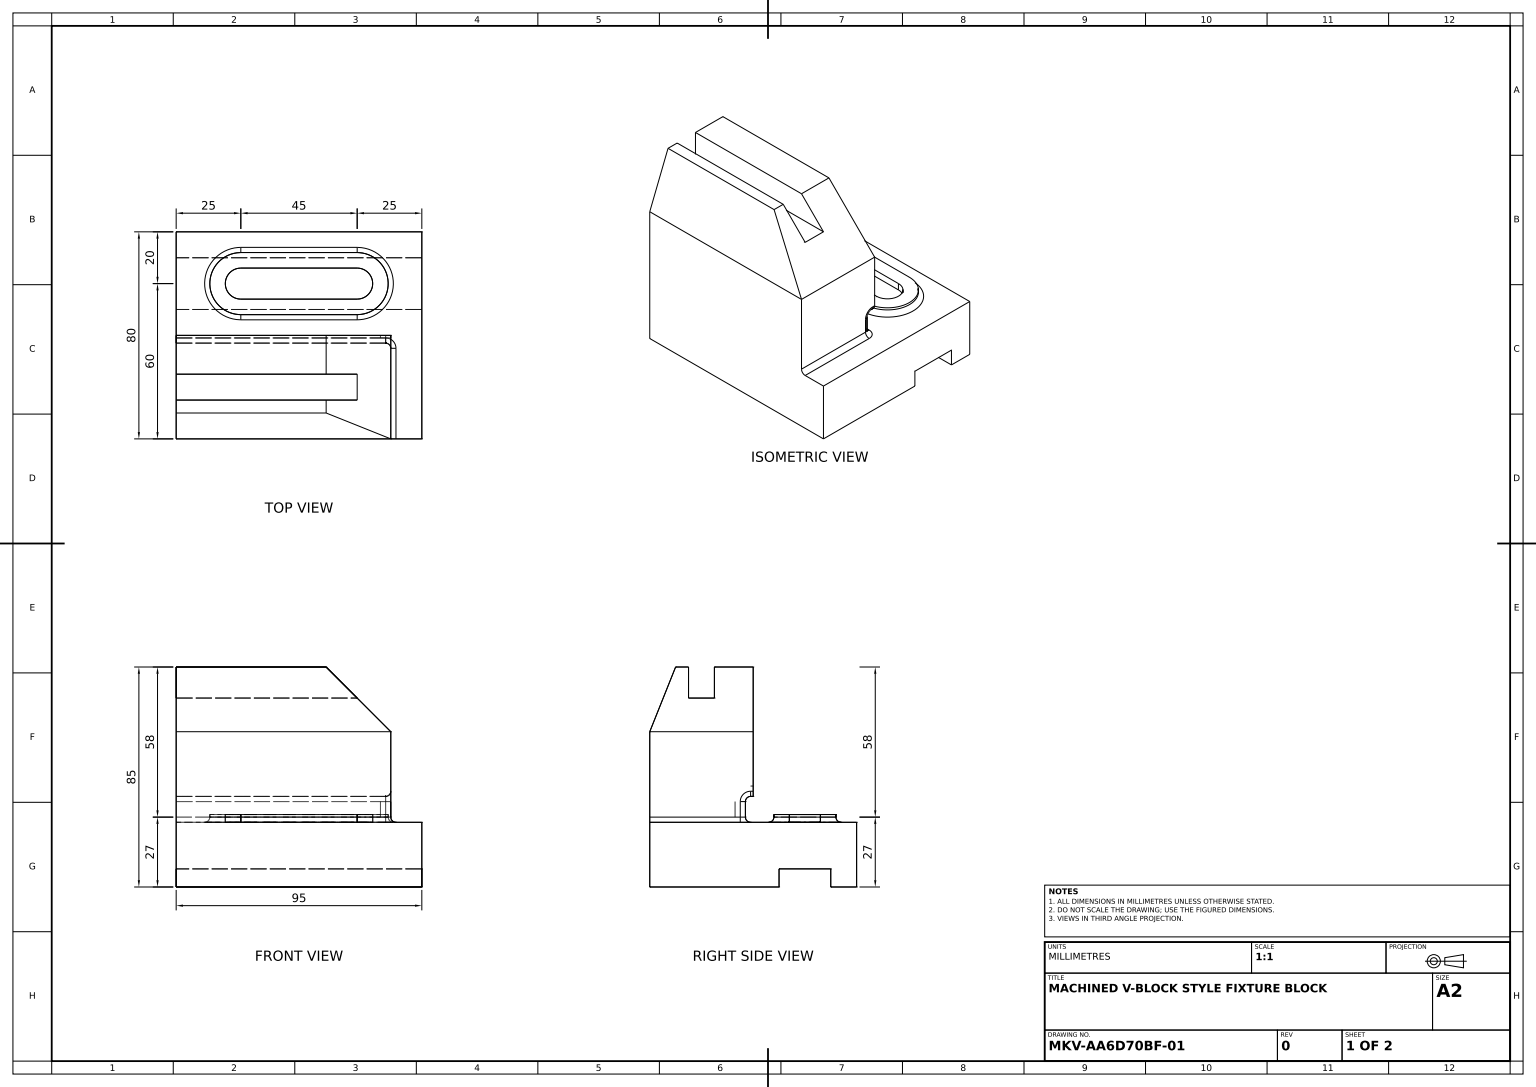
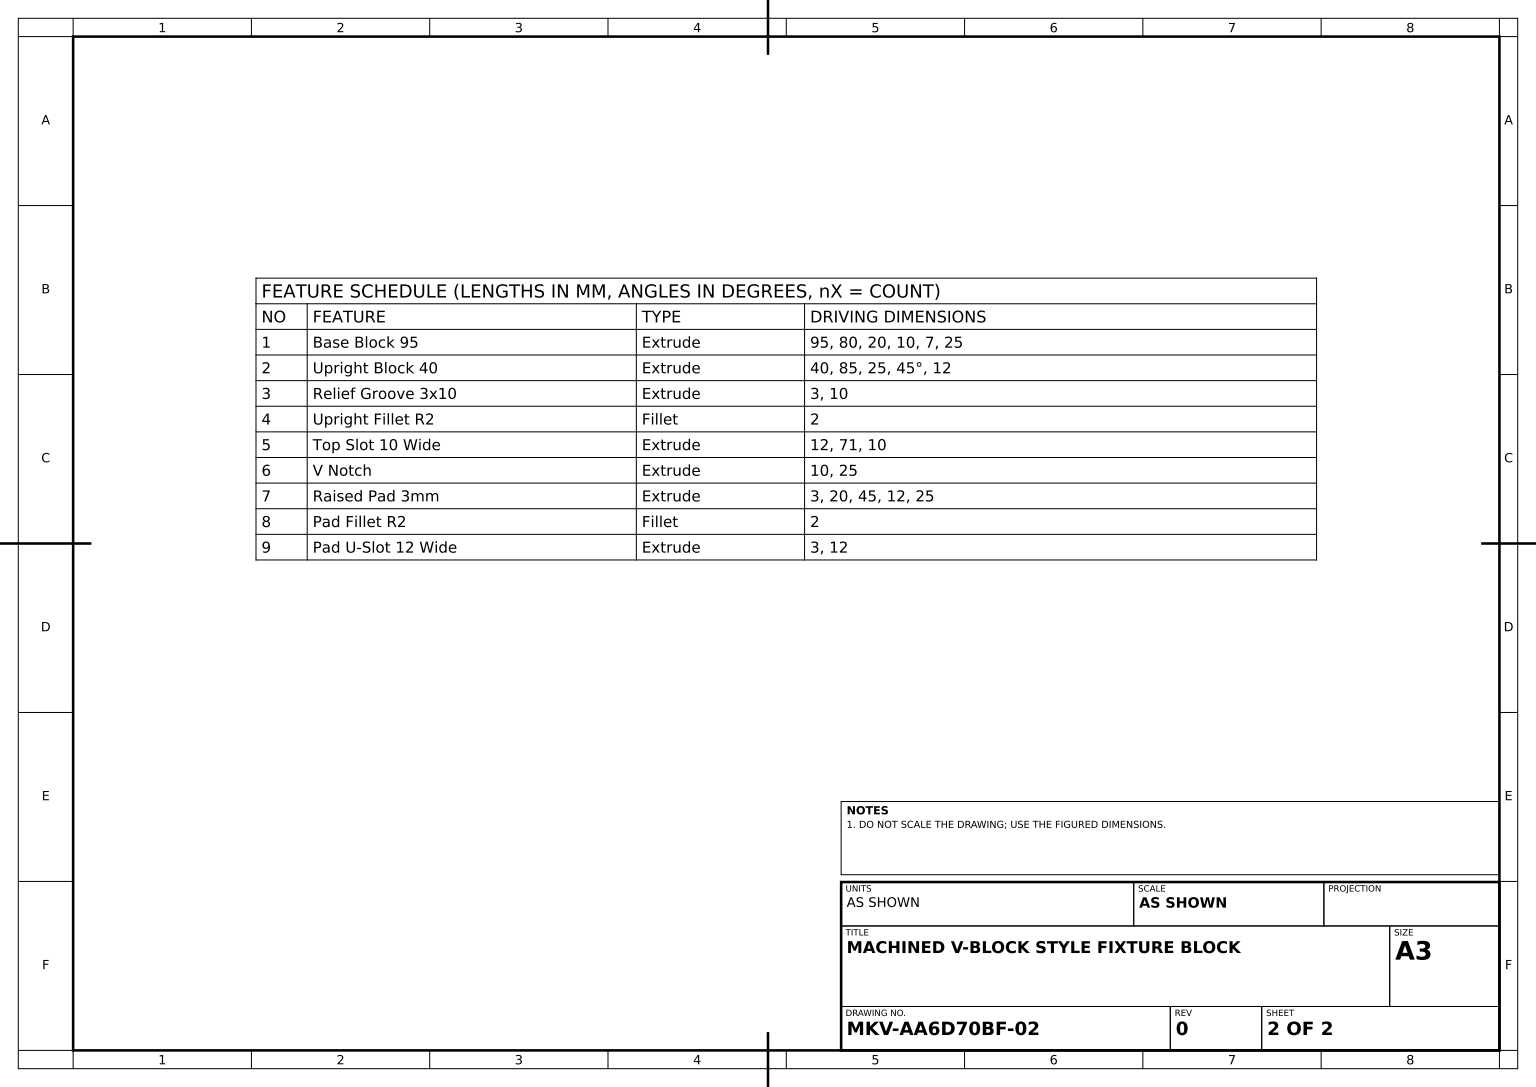
from build123d import *

# Parameters (mm, degrees)
BASE_BLOCK_95_DEPTH      = 47.5
UPRIGHT_BLOCK_40_DEPTH   = 40
RELIEF_GROOVE_SKETCH_W   = 3
RELIEF_GROOVE_SKETCH_H   = 10
RELIEF_GROOVE_3X10_DEPTH = 144.227092409
UPRIGHT_FILLET_R2_R      = 2
TOP_SLOT_SKETCH_W        = 71
TOP_SLOT_SKETCH_H        = 10
TOP_SLOT_10_WIDE_DEPTH   = 12
V_NOTCH_DEPTH            = 151.499169433
RAISED_PAD_3MM_DEPTH     = 3
PAD_FILLET_R2_R          = 2
PAD_U_SLOT_12_WIDE_DEPTH = 3


with BuildPart() as part:
    # Base Profile Sketch → Base Block 95 (new, symmetric)
    with BuildSketch(Plane(origin=(0, 0, 0), x_dir=(0, 0, -1), z_dir=(1, 0, 0))):
        Polygon((0, 0), (50, 0), (50, 7), (70, 7), (70, 0), (80, 0), (80, 25), (0, 25), align=None)
    extrude(amount=BASE_BLOCK_95_DEPTH, both=True)

    # Upright Profile Sketch → Upright Block 40 (add)
    with BuildSketch(Plane.XY):
        Polygon((-47.5, 25), (-47.5, 85), (10.5, 85), (35.5, 60), (35.5, 25), align=None)
    extrude(amount=-UPRIGHT_BLOCK_40_DEPTH)

    # Relief Groove Sketch → Relief Groove 3x10 (cut, through all)
    with BuildSketch(Plane(origin=(35.5, 0, 0), x_dir=(0, 0, -1), z_dir=(1, 0, 0))):
        with Locations((38.5, 30)):
            Rectangle(RELIEF_GROOVE_SKETCH_W, RELIEF_GROOVE_SKETCH_H)
    extrude(amount=-RELIEF_GROOVE_3X10_DEPTH, mode=Mode.SUBTRACT)

    # Upright Fillet R2
    upright_fillet_r2_edges = [part.edges().sort_by_distance(p)[0] for p in [
        (35.5, 25, -18.5),
        (-6, 25, -37),
        (-6, 35, -37),
        (35.5, 35, -38.5),
        (35.5, 30, -37),
    ]]
    fillet(upright_fillet_r2_edges, radius=UPRIGHT_FILLET_R2_R)

    # Top Slot Sketch → Top Slot 10 Wide (cut)
    with BuildSketch(Plane(origin=(0, 85, 0), x_dir=(1, 0, 0), z_dir=(0, 1, 0))):
        with Locations((-12, 20)):
            Rectangle(TOP_SLOT_SKETCH_W, TOP_SLOT_SKETCH_H)
    extrude(amount=-TOP_SLOT_10_WIDE_DEPTH, mode=Mode.SUBTRACT)

    # V Notch Sketch → V Notch (cut, through all)
    with BuildSketch(Plane.ZY.offset(47.5)):
        Polygon((0, 60), (0, 85), (-10, 85), align=None)
    extrude(amount=-V_NOTCH_DEPTH, mode=Mode.SUBTRACT)

    # Raised Pad Sketch → Raised Pad 3mm (add)
    with BuildSketch(Plane(origin=(0, 25, 0), x_dir=(1, 0, 0), z_dir=(0, 1, 0))):
        with BuildLine():
            Line((-22.5, 72), (22.5, 72))
            ThreePointArc((22.5, 72), (34.5, 60), (22.5, 48))
            Line((22.5, 48), (-22.5, 48))
            ThreePointArc((-22.5, 48), (-34.5, 60), (-22.5, 72))
        make_face()
    extrude(amount=RAISED_PAD_3MM_DEPTH)

    # Pad Fillet R2
    pad_fillet_r2_edges = [part.edges().sort_by_distance(p)[0] for p in [
        (-34.5, 25, -60),
        (0, 25, -48),
        (34.5, 25, -60),
        (0, 25, -72),
    ]]
    fillet(pad_fillet_r2_edges, radius=PAD_FILLET_R2_R)

    # Pad Slot Sketch → Pad U-Slot 12 Wide (cut)
    with BuildSketch(Plane(origin=(0, 28, 0), x_dir=(1, 0, 0), z_dir=(0, 1, 0))):
        with BuildLine():
            Line((-22.5, 66), (22.5, 66))
            ThreePointArc((22.5, 66), (28.5, 60), (22.5, 54))
            Line((22.5, 54), (-22.5, 54))
            ThreePointArc((-22.5, 54), (-28.5, 60), (-22.5, 66))
        make_face()
    extrude(amount=-PAD_U_SLOT_12_WIDE_DEPTH, mode=Mode.SUBTRACT)


solid = part.part
